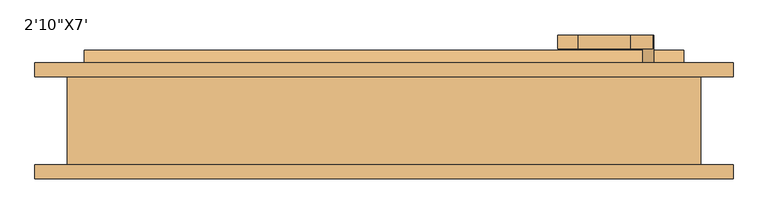
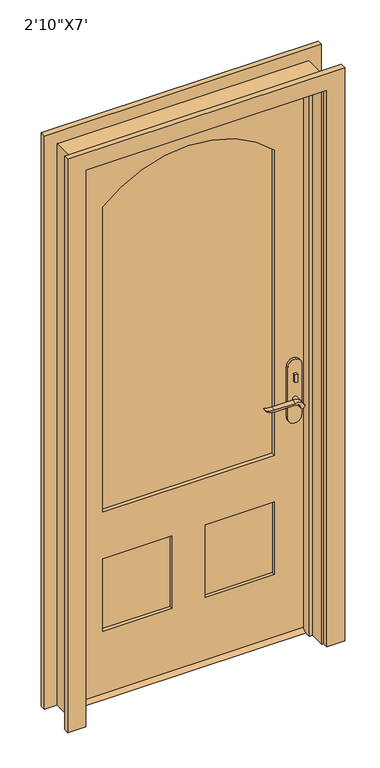
"""IFC4 building model written with IfcOpenShell, lengths in millimetres: door geometry."""

from ifc_helpers import new_model, si_unit, point, frame, frame_2d, origin, place, context, project, spatial, polyline, circle_curve, trimmed, segment, composite_curve, outline, extrude, faceted_brep, source, transform, mapped, element, save


def door_346b4a94(model_context):
    return source(origin(), model_context, "Body", "SolidModel", [
        extrude(outline(polyline([(38.025, 15.0), (73.025, 15.0), (98.425, 0.0), (12.625, 0.0), (38.025, 15.0)])), frame((-431.8, 0.0, 0.0), z_axis=(1.0, 0.0, 0.0), x_axis=(0.0, 1.0, 0.0)), (0.0, 0.0, 1.0), 863.6),
        extrude(outline(polyline([(385.6, 5.325), (375.6, 5.325), (375.6, 15.325), (385.6, 15.325), (385.6, 5.325)])), frame((0.0, 0.0, 981.9), z_axis=(0.0, 0.0, 1.0), x_axis=(1.0, 0.0, 0.0)), (0.0, 0.0, 1.0), 30.0),
        extrude(outline(composite_curve([segment(trimmed(circle_curve(frame_2d((996.9, 380.6)), 8.0), [point((996.9, 372.6))], [point((996.9, 388.6))], False, "CARTESIAN"), True, "CONTINUOUS"), segment(trimmed(circle_curve(frame_2d((996.9, 380.6)), 8.0), [point((996.9, 388.6))], [point((996.9, 372.6))], False, "CARTESIAN"), True, "CONTINUOUS")], self_intersect=False)), frame((0.0, 70.325, 0.0), z_axis=(0.0, 1.0, 0.0), x_axis=(0.0, 0.0, 1.0)), (0.0, 0.0, 1.0), 10.0),
        extrude(outline(composite_curve([segment(trimmed(circle_curve(frame_2d((897.1555521, 356.9324871)), 37.2832219), [point((919.0523287, 387.1081363))], [point((934.4, 355.2325667))], False, "CARTESIAN"), True, "CONTINUOUS"), segment(polyline([(934.4, 355.2325667), (934.4, 278.9564091)]), True, "CONTINUOUS"), segment(trimmed(circle_curve(frame_2d((1017.6850638, 279.0227909)), 83.2850902), [point((934.4, 278.9564091))], [point((939.4, 250.6))], True, "CARTESIAN"), True, "CONTINUOUS"), segment(polyline([(939.4, 250.6), (936.6135558, 250.6)]), True, "CONTINUOUS"), segment(trimmed(circle_curve(frame_2d((986.6709207, 282.5396612)), 59.3791355), [point((936.6135558, 250.6))], [point((927.4, 278.9564091))], False, "CARTESIAN"), True, "CONTINUOUS"), segment(polyline([(927.4, 278.9564091), (927.4, 355.2138099)]), True, "CONTINUOUS"), segment(trimmed(circle_curve(frame_2d((909.2738613, 355.2138099)), 18.1261387), [point((927.4, 355.2138099))], [point((914.4, 372.6))], True, "CARTESIAN"), True, "CONTINUOUS"), segment(trimmed(circle_curve(frame_2d((914.4, 380.6)), 8.0), [point((914.4, 372.6))], [point((919.0523287, 387.1081363))], False, "CARTESIAN"), True, "CONTINUOUS")], self_intersect=False)), frame((0.0, -34.675, 0.0), z_axis=(0.0, 1.0, 0.0), x_axis=(0.0, 0.0, 1.0)), (0.0, 0.0, 1.0), 20.0),
        extrude(outline(composite_curve([segment(trimmed(circle_curve(frame_2d((914.4, 380.6)), 8.0), [point((914.3999903, 372.6))], [point((919.0523287, 387.1081363))], False, "CARTESIAN"), True, "CONTINUOUS"), segment(trimmed(circle_curve(frame_2d((897.1555521, 356.9324871)), 37.2832219), [point((919.0523287, 387.1081363))], [point((934.4, 355.2325667))], False, "CARTESIAN"), True, "CONTINUOUS"), segment(polyline([(934.4, 355.2325667), (934.4, 278.9564091)]), True, "CONTINUOUS"), segment(trimmed(circle_curve(frame_2d((1017.6850638, 279.0227909)), 83.2850902), [point((934.4, 278.9564091))], [point((939.4, 250.6))], True, "CARTESIAN"), True, "CONTINUOUS"), segment(polyline([(939.4, 250.6), (936.6135558, 250.6)]), True, "CONTINUOUS"), segment(trimmed(circle_curve(frame_2d((986.6709207, 282.5396612)), 59.3791355), [point((936.6135558, 250.6))], [point((927.4, 278.9564091))], False, "CARTESIAN"), True, "CONTINUOUS"), segment(polyline([(927.4, 278.9564091), (927.4, 355.2138122)]), True, "CONTINUOUS"), segment(trimmed(circle_curve(frame_2d((909.2738682, 355.2138122)), 18.1261318), [point((927.4, 355.2138122))], [point((914.3999903, 372.6))], True, "CARTESIAN"), True, "CONTINUOUS")], self_intersect=False)), frame((0.0, 100.325, 0.0), z_axis=(0.0, 1.0, 0.0), x_axis=(0.0, 0.0, 1.0)), (0.0, 0.0, 1.0), 20.0),
        extrude(outline(composite_curve([segment(trimmed(circle_curve(frame_2d((914.4, 380.6)), 8.0), [point((914.4, 372.6))], [point((914.4, 388.6))], False, "CARTESIAN"), True, "CONTINUOUS"), segment(trimmed(circle_curve(frame_2d((914.4, 380.6)), 8.0), [point((914.4, 388.6))], [point((914.4, 372.6))], False, "CARTESIAN"), True, "CONTINUOUS")], self_intersect=False)), frame((0.0, -14.675, 0.0), z_axis=(0.0, 1.0, 0.0), x_axis=(0.0, 0.0, 1.0)), (0.0, 0.0, 1.0), 30.0),
        extrude(outline(composite_curve([segment(trimmed(circle_curve(frame_2d((914.4, 380.6)), 8.0), [point((914.4, 372.6))], [point((914.4, 388.6))], False, "CARTESIAN"), True, "CONTINUOUS"), segment(trimmed(circle_curve(frame_2d((914.4, 380.6)), 8.0), [point((914.4, 388.6))], [point((914.4, 372.6))], False, "CARTESIAN"), True, "CONTINUOUS")], self_intersect=False)), frame((0.0, 70.325, 0.0), z_axis=(0.0, 1.0, 0.0), x_axis=(0.0, 0.0, 1.0)), (0.0, 0.0, 1.0), 30.0),
        extrude(outline(composite_curve([segment(polyline([(844.4, 405.6), (1039.4, 405.6)]), True, "CONTINUOUS"), segment(trimmed(circle_curve(frame_2d((1039.4, 380.6)), 25.0), [point((1039.4, 405.6))], [point((1039.4, 355.6))], False, "CARTESIAN"), True, "CONTINUOUS"), segment(polyline([(1039.4, 355.6), (844.4, 355.6)]), True, "CONTINUOUS"), segment(trimmed(circle_curve(frame_2d((844.4, 380.6)), 25.0), [point((844.4, 355.6))], [point((844.4, 405.6))], False, "CARTESIAN"), True, "CONTINUOUS")], self_intersect=False)), frame((0.0, 15.325, 0.0), z_axis=(0.0, 1.0, 0.0), x_axis=(0.0, 0.0, 1.0)), (0.0, 0.0, 1.0), 10.0),
        extrude(outline(composite_curve([segment(polyline([(844.4, 405.6), (1039.4, 405.6)]), True, "CONTINUOUS"), segment(trimmed(circle_curve(frame_2d((1039.4, 380.6)), 25.0), [point((1039.4, 405.6))], [point((1039.4, 355.6))], False, "CARTESIAN"), True, "CONTINUOUS"), segment(polyline([(1039.4, 355.6), (844.4, 355.6)]), True, "CONTINUOUS"), segment(trimmed(circle_curve(frame_2d((844.4, 380.6)), 25.0), [point((844.4, 355.6))], [point((844.4, 405.6))], False, "CARTESIAN"), True, "CONTINUOUS")], self_intersect=False)), frame((0.0, 60.325, 0.0), z_axis=(0.0, 1.0, 0.0), x_axis=(0.0, 0.0, 1.0)), (0.0, 0.0, 1.0), 10.0),
        faceted_brep([(456.8, 60.325, 0.0), (456.8, -66.675, 0.0), (431.8, -66.675, 0.0), (431.8, -9.6, 0.0), (419.1, -9.6, 0.0), (419.1, 25.325, 0.0), (431.8, 25.325, 0.0), (431.8, 60.325, 0.0), (456.8, 60.325, 2158.6), (456.8, -66.675, 2158.6), (-456.8, -66.675, 2158.6), (-456.8, -66.675, 0.0), (-431.8, -66.675, 0.0), (-431.8, -66.675, 2133.6), (431.8, -66.675, 2133.6), (431.8, -9.6, 2133.6), (-431.8, -9.6, 2133.6), (-431.8, -9.6, 0.0), (-419.1, -9.6, 0.0), (-419.1, -9.6, 2120.9), (419.1, -9.6, 2120.9), (419.1, 25.325, 2120.9), (-419.1, 25.325, 2120.9), (-419.1, 25.325, 0.0), (-431.8, 25.325, 0.0), (-431.8, 25.325, 2133.6), (431.8, 25.325, 2133.6), (431.8, 60.325, 2133.6), (-431.8, 60.325, 2133.6), (-431.8, 60.325, 0.0), (-456.8, 60.325, 0.0), (-456.8, 60.325, 2158.6)], [[[0, 1, 2, 3, 4, 5, 6, 7]], [[1, 0, 8, 9]], [[2, 1, 9, 10, 11, 12, 13, 14]], [[3, 2, 14, 15]], [[4, 3, 15, 16, 17, 18, 19, 20]], [[5, 4, 20, 21]], [[6, 5, 21, 22, 23, 24, 25, 26]], [[7, 6, 26, 27]], [[0, 7, 27, 28, 29, 30, 31, 8]], [[9, 8, 31, 10]], [[15, 14, 13, 16]], [[21, 20, 19, 22]], [[27, 26, 25, 28]], [[30, 29, 24, 23, 18, 17, 12, 11]], [[10, 31, 30, 11]], [[16, 13, 12, 17]], [[22, 19, 18, 23]], [[28, 25, 24, 29]]]),
        extrude(outline(polyline([(2133.6, -431.8), (15.0, -431.8), (15.0, 431.8), (2133.6, 431.8), (2133.6, -431.8)]), holes=[composite_curve([segment(polyline([(713.4, -311.8), (1885.95, -311.8)]), True, "CONTINUOUS"), segment(trimmed(circle_curve(frame_2d((1566.6970866, 0.0)), 446.2529134), [point((1885.95, -311.8))], [point((1885.95, 311.8))], True, "CARTESIAN"), True, "CONTINUOUS"), segment(polyline([(1885.95, 311.8), (713.4, 311.8), (713.4, -311.8)]), True, "CONTINUOUS")], self_intersect=False), polyline([(533.4, -60.325), (255.0, -60.325), (255.0, -311.8), (533.4, -311.8), (533.4, -60.325)]), polyline([(533.4, 311.8), (255.0, 311.8), (255.0, 60.325), (533.4, 60.325), (533.4, 311.8)])]), frame((0.0, 25.325, 0.0), z_axis=(0.0, 1.0, 0.0), x_axis=(0.0, 0.0, 1.0)), (0.0, 0.0, 1.0), 35.0),
        extrude(outline(composite_curve([segment(polyline([(713.4, -311.8), (713.4, 311.8), (1885.95, 311.8)]), True, "CONTINUOUS"), segment(trimmed(circle_curve(frame_2d((1566.6970866, 0.0)), 446.2529134), [point((1885.95, 311.8))], [point((1885.95, -311.8))], False, "CARTESIAN"), True, "CONTINUOUS"), segment(polyline([(1885.95, -311.8), (713.4, -311.8)]), True, "CONTINUOUS")], self_intersect=False)), frame((0.0, 39.325, 0.0), z_axis=(0.0, 1.0, 0.0), x_axis=(0.0, 0.0, 1.0)), (0.0, 0.0, 1.0), 7.0),
        extrude(outline(polyline([(-60.325, 36.9916667), (-311.8, 36.9916667), (-311.8, 48.6583333), (-60.325, 48.6583333), (-60.325, 36.9916667)])), frame((0.0, 0.0, 256.3), z_axis=(0.0, 0.0, 1.0), x_axis=(1.0, 0.0, 0.0)), (0.0, 0.0, 1.0), 277.1),
        extrude(outline(polyline([(311.8, 36.9916667), (60.325, 36.9916667), (60.325, 48.6583333), (311.8, 48.6583333), (311.8, 36.9916667)])), frame((0.0, 0.0, 255.0), z_axis=(0.0, 0.0, 1.0), x_axis=(1.0, 0.0, 0.0)), (0.0, 0.0, 1.0), 278.4),
        extrude(outline(polyline([(0.0, -503.15), (0.0, -438.15), (2139.95, -438.15), (2139.95, 438.15), (0.0, 438.15), (0.0, 503.15), (2204.95, 503.15), (2204.95, -503.15), (0.0, -503.15)])), frame((0.0, 60.325, 0.0), z_axis=(0.0, 1.0, 0.0), x_axis=(0.0, 0.0, 1.0)), (0.0, 0.0, 1.0), 20.0),
        extrude(outline(polyline([(0.0, -503.15), (0.0, -438.15), (2139.95, -438.15), (2139.95, 438.15), (0.0, 438.15), (0.0, 503.15), (2204.95, 503.15), (2204.95, -503.15), (0.0, -503.15)])), frame((0.0, -86.675, 0.0), z_axis=(0.0, 1.0, 0.0), x_axis=(0.0, 0.0, 1.0)), (0.0, 0.0, 1.0), 20.0),
    ])


if __name__ == "__main__":
    model = new_model("IFC4")
    model_context = context("Model", 3, world=origin())
    ifc_project = project(units=[si_unit("LENGTHUNIT", "METRE", prefix="MILLI")], contexts=[model_context])
    site = spatial("IfcSite", under=ifc_project)
    building = spatial("IfcBuilding", under=site)
    placement = place(None, origin())
    door_shape = door_346b4a94(model_context)
    element("IfcDoor", 1, ObjectType="2'10\"X7'", at=placement, inside=building, context=model_context, shape_type="MappedRepresentation", body=[
        mapped(door_shape, transform((0.0, 0.0, 0.0), x_axis=(1.0, 0.0, 0.0), y_axis=(0.0, 1.0, 0.0), z_axis=(0.0, 0.0, 1.0))),
    ])
    save(model, "model.ifc")

# Revit data of these elements
# Type "2'10\"X7'"
#   Type Mark = "9"
#   Assembly Code = "B2030100"
#   Analytic Construction = "French door, wood frame with single glass"
#   Threshold Offset [instance default] = 0' - 0.59055"
#   Thickness = 0' - 1.37795"
#   Thermal Resistance (R) = 1.0696 (h·ft²·°F)/BTU
#   Swing Angle [instance default] = 90.00°
#   Stiles = 0' - 4.72441"
#   Rough Width = 2' - 11.9685"
#   Rough Height = 7' - 0.98425"
#   Radius = 1' - 5.56901"
#   Lock Rail = 0' - 7.08661"
#   Height = 7' - 0"
#   Width = 2' - 10"
#   Heat Transfer Coefficient (U) = 0.9350 BTU/(h·ft²·°F)
#   Door Offset [instance default] = 0' - 0"
#   Bottom Rail = 0' - 9.44882"
#   Threshold [instance default] = yes
#   Function = 1
#   Exterior Trim [instance default] = yes
#   Trim Material = Cherry
#   Threshold Material = Cherry
#   Panel Material = Cherry
#   Glazing = Glass
#   Frame Material = Cherry
#   Door Handle Material = Aluminum
#   Visual Light Transmittance = 0
#   Solar Heat Gain Coefficient = 0
#   Wall Closure = (empty or 0)
#   Construction Type = (empty or 0)
# Element 1 (IfcDoor, "2'10\"X7'")
#   Materials on its faces: "Cherry", "Aluminum", "Glass"
# Materials
#   "Cherry": class "Wood", colour RGB 226 177 128, transparency 0, Description = "Prunus Serotina", Cost = 0
#   "Glass": class "Glass", colour RGB 0 128 192, transparency 0.75, Description = "Soda Lime Glass", Cost = 0
#   "Aluminum": class "Metal", colour RGB 247 247 247, transparency 0, Description = "Aluminum 6061", Cost = 0
